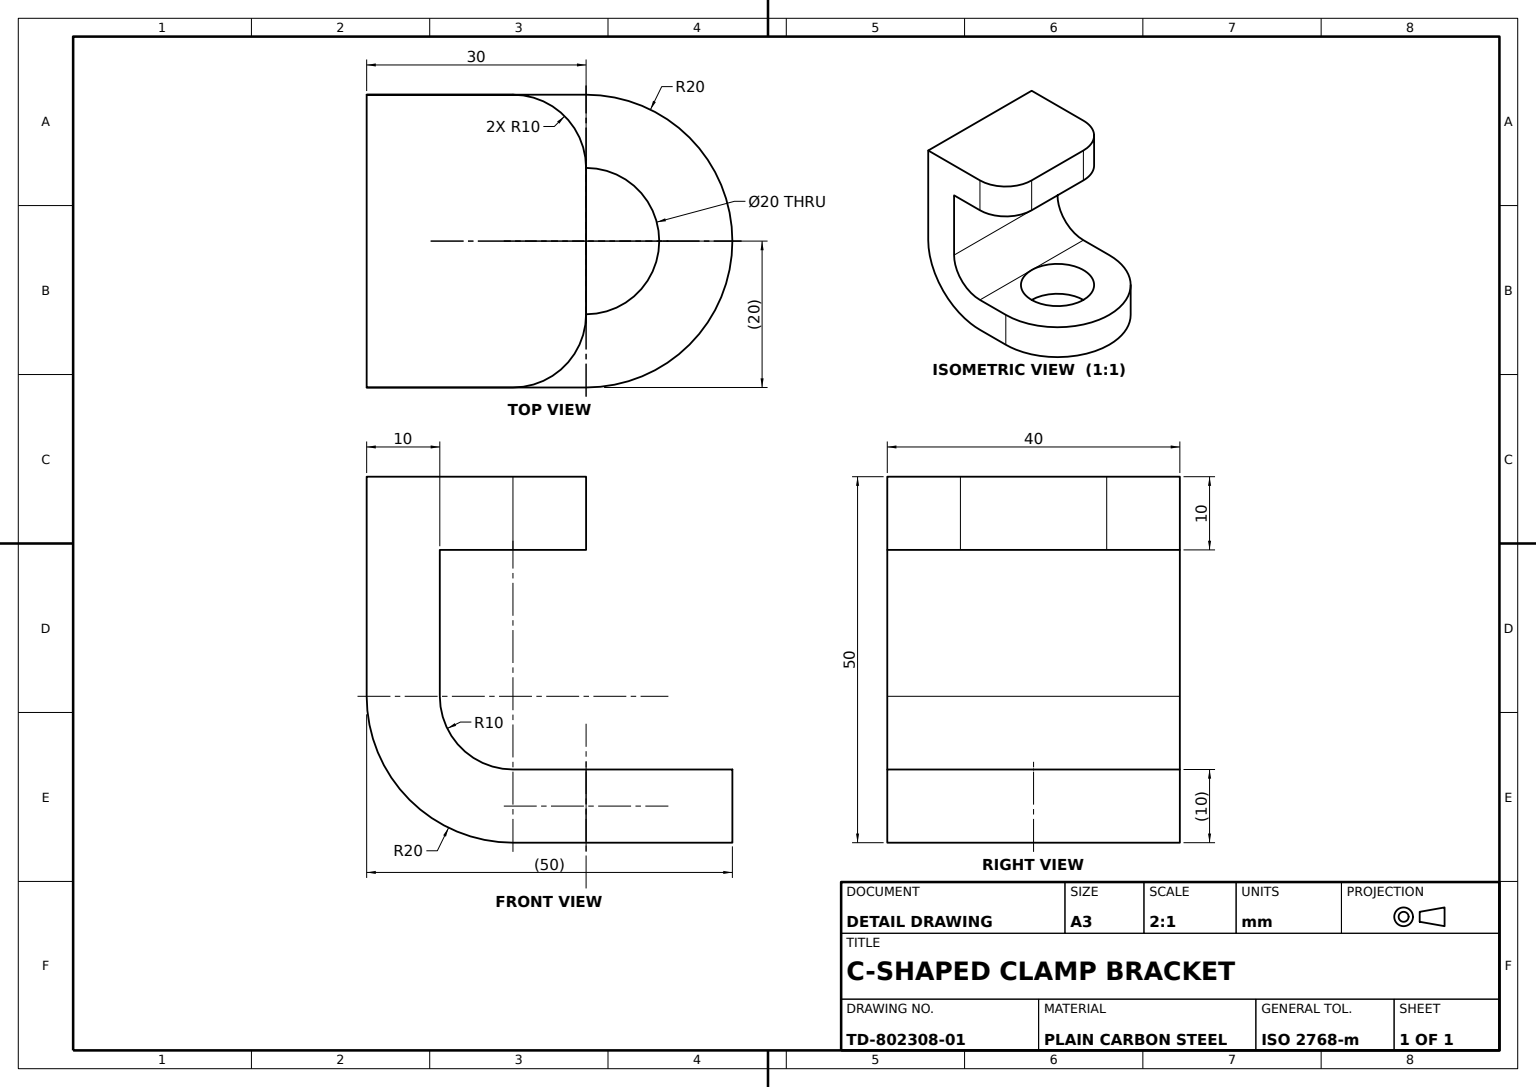
from build123d import *

# Parameters (mm, degrees)
BRACKET_BODY_DEPTH      = 20
EDGE_FILLETS_R10_R      = 10
MOUNTING_HOLE_SKETCH_R  = 10
MOUNTING_HOLE_CUT_DEPTH = 10


with BuildPart() as part:
    # Bracket Profile Sketch → Bracket Body (new, symmetric)
    with BuildSketch(Plane.XY):
        with BuildLine():
            Line((0, 20), (0, 50))
            Line((0, 50), (30, 50))
            Line((30, 50), (30, 40))
            Line((30, 40), (10, 40))
            Line((10, 40), (10, 20))
            ThreePointArc((10, 20), (12.928932188, 12.928932188), (20, 10))
            Line((20, 10), (50, 10))
            Line((50, 10), (50, 0))
            Line((50, 0), (20, 0))
            ThreePointArc((20, 0), (5.857864376, 5.857864376), (0, 20))
        make_face()
    extrude(amount=BRACKET_BODY_DEPTH, both=True)

    # Edge Fillets R10
    edge_fillets_r10_edges = [part.edges().sort_by_distance(p)[0] for p in [
        (30, 45, -20),
        (30, 45, 20),
    ]]
    fillet(edge_fillets_r10_edges, radius=EDGE_FILLETS_R10_R)

    # Mounting Hole Sketch → Mounting Hole Cut (cut)
    with BuildSketch(Plane.XZ):
        with BuildLine():
            Line((50, 20), (30, 20))
            ThreePointArc((30, 20), (44.142135624, 14.142135624), (50, 0))
            Line((50, 0), (50, 20))
        make_face()
        with BuildLine():
            Line((50, -20), (50, 0))
            ThreePointArc((50, 0), (44.142135624, -14.142135624), (30, -20))
            Line((30, -20), (50, -20))
        make_face()
        with Locations(Location((30, 0, 0), (0, 0, 180))):
            Circle(MOUNTING_HOLE_SKETCH_R)
    extrude(amount=-MOUNTING_HOLE_CUT_DEPTH, mode=Mode.SUBTRACT)


solid = part.part
